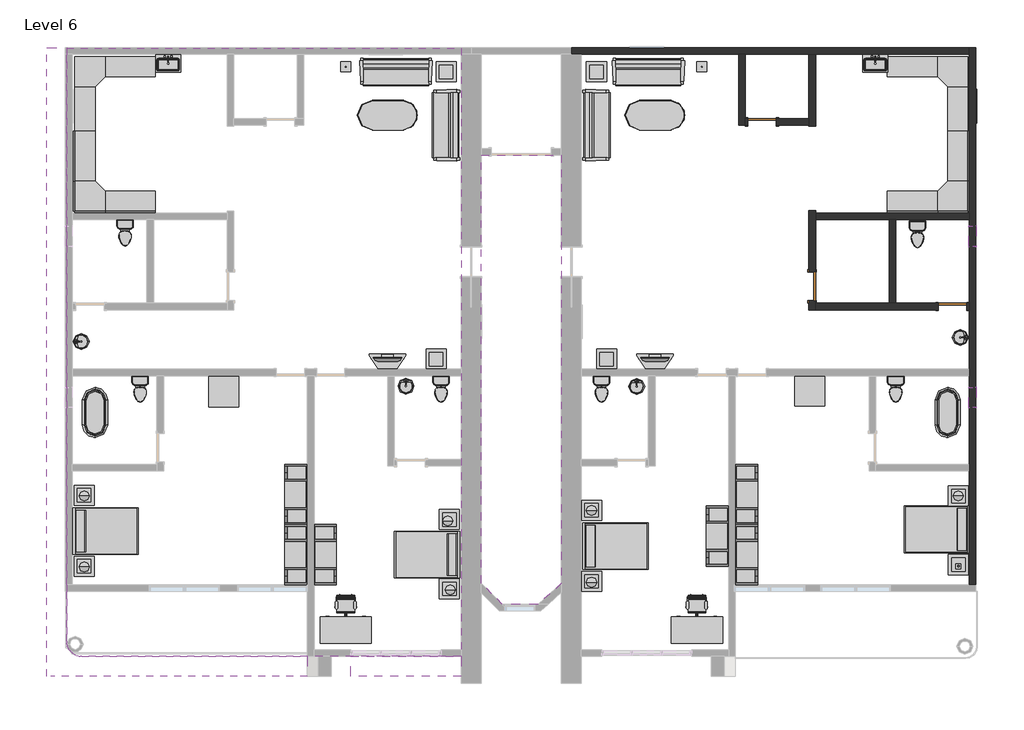
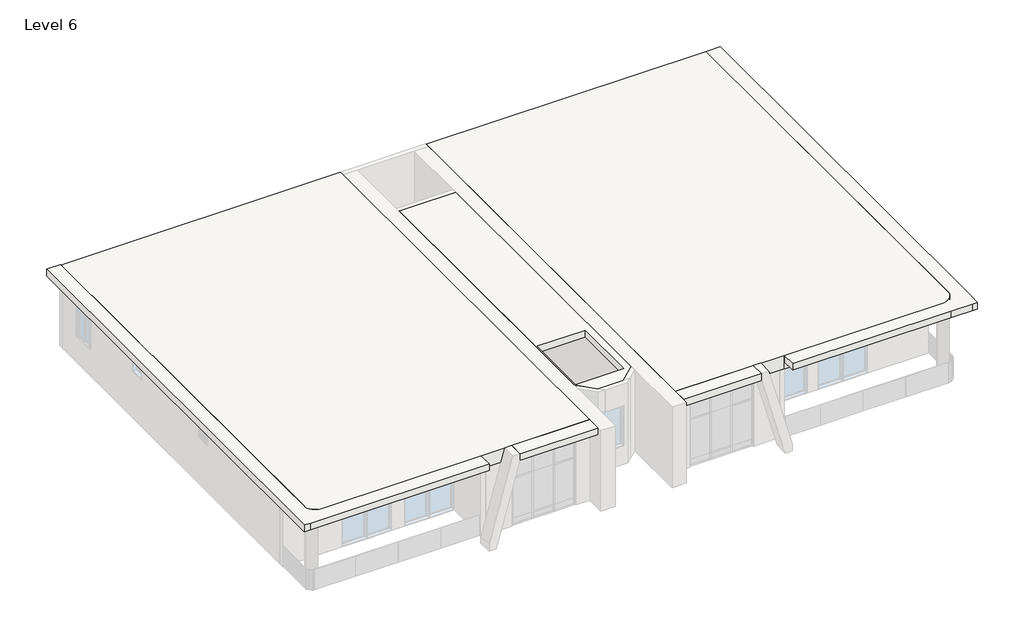
# One storey, part 3 of 3: 42 furniture elements, 14 flow terminals, 10 light fixtures, 9 walls, 4 slabs, 3 doors, 3 windows.
"""IFC4 building model written with IfcOpenShell, lengths in millimetres."""

from ifc_helpers import new_model, si_unit, point, frame, frame_2d, origin, place, context, project, spatial, polyline, circle_curve, trimmed, segment, composite_curve, outline, extrude, faceted_brep, transform, mapped, element, save
from components import door_2703ae13, door_10fd3a06, flow_terminal_38af2918, flow_terminal_d49f872f, toilet_domestic_3d_toilet_domestic_3d_f7549cf7, toilet_domestic_3d_toilet_domestic_3d_183bbd19, flow_terminal_b374fae2, furniture_07436f11, furniture_096e7f55, chair_task_arms_chair_task_arms_fa5a08ef, furniture_072f6425, furniture_cf0b6580, furniture_aff9b2fb, furniture_56245f3a, tv_stand_tv_stand_6ce107e5, furniture_b5c51a22, furniture_2c34a4f9, furniture_4d44e21c, furniture_45e3acac, light_fixture_100w_120v_8564026f, table_lamp_hemispheric_60w_120v_02721d88, window_0038ecf3, window_54100e87

model = new_model("IFC4")

# Units and contexts
model_context = context("Model", 3, world=origin())
ifc_project = project(units=[si_unit("LENGTHUNIT", "METRE", prefix="MILLI")], contexts=[model_context])

# Site, building, storey
site = spatial("IfcSite", under=ifc_project)
building = spatial("IfcBuilding", under=site)
storey = spatial("IfcBuildingStorey", under=building, Name="Level 6", Elevation=18288.0)

# Doors
placement = place(None, origin())
door_shape = door_2703ae13(model_context)
element("IfcDoor", 1, ObjectType="Door-Single-Panel.0001 : 34\" x 80\"", at=placement, inside=storey, context=model_context, shape_type="MappedRepresentation", body=[
    mapped(door_shape, transform((2522.0012296, 9464.0758558, 18288.0), x_axis=(-1.0, 0.0, 0.0), y_axis=(0.0, -1.0, 0.0), z_axis=(0.0, 0.0, 1.0))),
])
door_2_shape = door_10fd3a06(model_context)
element("IfcDoor", 2, ObjectType="Door-Single-Panel.0001 : 34\" x 80\"", at=placement, inside=storey, context=model_context, shape_type="MappedRepresentation", body=[
    mapped(door_2_shape, transform((8313.2012296, 3850.6758558, 18288.0), x_axis=(1.0, 0.0, 0.0), y_axis=(0.0, 1.0, 0.0), z_axis=(0.0, 0.0, 1.0))),
])
element("IfcDoor", 3, ObjectType="Door-Single-Panel.0001 : 34\" x 80\"", at=placement, inside=storey, context=model_context, shape_type="MappedRepresentation", body=[
    mapped(door_2_shape, transform((4046.0012296, 4460.2758558, 18288.0), x_axis=(0.0, -1.0, 0.0), y_axis=(1.0, 0.0, 0.0), z_axis=(0.0, 0.0, 1.0))),
])

# Flow terminals
flow_terminal_shape = flow_terminal_38af2918(model_context)
element("IfcFlowTerminal", 4, ObjectType="Sink Kitchen-Single : 30\" x 21\"", at=placement, inside=storey, context=model_context, shape_type="MappedRepresentation", body=[
    mapped(flow_terminal_shape, transform((-15540.388011, 11239.7304546, 18288.0), x_axis=(1.0, 0.0, 0.0), y_axis=(0.0, 1.0, 0.0), z_axis=(0.0, 0.0, 1.0))),
])
element("IfcFlowTerminal", 5, ObjectType="Sink Kitchen-Single : 30\" x 21\"", at=placement, inside=storey, context=model_context, shape_type="MappedRepresentation", body=[
    mapped(flow_terminal_shape, transform((5948.011989, 11239.7304546, 18288.0), x_axis=(1.0, 0.0, 0.0), y_axis=(0.0, 1.0, 0.0), z_axis=(0.0, 0.0, 1.0))),
])
flow_terminal_2_shape = flow_terminal_d49f872f(model_context)
element("IfcFlowTerminal", 6, ObjectType="Sink Vanity-Round : 19\" x 19\"", at=placement, inside=storey, context=model_context, shape_type="MappedRepresentation", body=[
    mapped(flow_terminal_2_shape, transform((-18084.6070794, 2687.2241152, 18288.0), x_axis=(0.0, 1.0, 0.0), y_axis=(-1.0, 0.0, 0.0), z_axis=(0.0, 0.0, 1.0))),
])
element("IfcFlowTerminal", 7, ObjectType="Sink Vanity-Round : 19\" x 19\"", at=placement, inside=storey, context=model_context, shape_type="MappedRepresentation", body=[
    mapped(flow_terminal_2_shape, transform((8462.2249463, 3007.5275963, 18288.0), x_axis=(0.0, -1.0, 0.0), y_axis=(1.0, 0.0, 0.0), z_axis=(0.0, 0.0, 1.0))),
])
element("IfcFlowTerminal", 8, ObjectType="Sink Vanity-Round : 19\" x 19\"", at=placement, inside=storey, context=model_context, shape_type="MappedRepresentation", body=[
    mapped(flow_terminal_2_shape, transform((-8395.050511, 1341.8921141, 18288.0), x_axis=(1.0, 0.0, 0.0), y_axis=(0.0, 1.0, 0.0), z_axis=(0.0, 0.0, 1.0))),
])
element("IfcFlowTerminal", 9, ObjectType="Sink Vanity-Round : 19\" x 19\"", at=placement, inside=storey, context=model_context, shape_type="MappedRepresentation", body=[
    mapped(flow_terminal_2_shape, transform((-1384.650511, 1331.0855344, 18288.0), x_axis=(1.0, 0.0, 0.0), y_axis=(0.0, 1.0, 0.0), z_axis=(0.0, 0.0, 1.0))),
])
toilet_domestic_3d_toilet_domestic_3d_shape = toilet_domestic_3d_toilet_domestic_3d_f7549cf7(model_context)
toilet_domestic_3d_toilet_domestic_3d_2_shape = toilet_domestic_3d_toilet_domestic_3d_183bbd19(model_context)
element("IfcFlowTerminal", 10, ObjectType="Toilet-Domestic-3D : Toilet-Domestic-3D", at=placement, inside=storey, context=model_context, shape_type="MappedRepresentation", body=[
    mapped(toilet_domestic_3d_toilet_domestic_3d_shape, transform((6586.0012296, 1247.7798284, 18288.0), x_axis=(1.0, 0.0, 0.0), y_axis=(0.0, 1.0, 0.0), z_axis=(0.0, 0.0, 1.0))),
    mapped(toilet_domestic_3d_toilet_domestic_3d_2_shape, transform((6586.0012296, 1247.7798284, 18288.0), x_axis=(1.0, 0.0, 0.0), y_axis=(0.0, 1.0, 0.0), z_axis=(0.0, 0.0, 1.0))),
])
element("IfcFlowTerminal", 11, ObjectType="Toilet-Domestic-3D : Toilet-Domestic-3D", at=placement, inside=storey, context=model_context, shape_type="MappedRepresentation", body=[
    mapped(toilet_domestic_3d_toilet_domestic_3d_shape, transform((-2354.7987704, 1247.7798284, 18288.0), x_axis=(1.0, 0.0, 0.0), y_axis=(0.0, 1.0, 0.0), z_axis=(0.0, 0.0, 1.0))),
    mapped(toilet_domestic_3d_toilet_domestic_3d_2_shape, transform((-2354.7987704, 1247.7798284, 18288.0), x_axis=(1.0, 0.0, 0.0), y_axis=(0.0, 1.0, 0.0), z_axis=(0.0, 0.0, 1.0))),
])
element("IfcFlowTerminal", 12, ObjectType="Toilet-Domestic-3D : Toilet-Domestic-3D", at=placement, inside=storey, context=model_context, shape_type="MappedRepresentation", body=[
    mapped(toilet_domestic_3d_toilet_domestic_3d_shape, transform((-16375.5987704, 1247.7798284, 18288.0), x_axis=(1.0, 0.0, 0.0), y_axis=(0.0, 1.0, 0.0), z_axis=(0.0, 0.0, 1.0))),
    mapped(toilet_domestic_3d_toilet_domestic_3d_2_shape, transform((-16375.5987704, 1247.7798284, 18288.0), x_axis=(1.0, 0.0, 0.0), y_axis=(0.0, 1.0, 0.0), z_axis=(0.0, 0.0, 1.0))),
])
element("IfcFlowTerminal", 13, ObjectType="Toilet-Domestic-3D : Toilet-Domestic-3D", at=placement, inside=storey, context=model_context, shape_type="MappedRepresentation", body=[
    mapped(toilet_domestic_3d_toilet_domestic_3d_shape, transform((-16832.7987704, 5997.5798284, 18288.0), x_axis=(1.0, 0.0, 0.0), y_axis=(0.0, 1.0, 0.0), z_axis=(0.0, 0.0, 1.0))),
    mapped(toilet_domestic_3d_toilet_domestic_3d_2_shape, transform((-16832.7987704, 5997.5798284, 18288.0), x_axis=(1.0, 0.0, 0.0), y_axis=(0.0, 1.0, 0.0), z_axis=(0.0, 0.0, 1.0))),
])
element("IfcFlowTerminal", 14, ObjectType="Toilet-Domestic-3D : Toilet-Domestic-3D", at=placement, inside=storey, context=model_context, shape_type="MappedRepresentation", body=[
    mapped(toilet_domestic_3d_toilet_domestic_3d_shape, transform((7246.4012296, 5946.7798284, 18288.0), x_axis=(1.0, 0.0, 0.0), y_axis=(0.0, 1.0, 0.0), z_axis=(0.0, 0.0, 1.0))),
    mapped(toilet_domestic_3d_toilet_domestic_3d_2_shape, transform((7246.4012296, 5946.7798284, 18288.0), x_axis=(1.0, 0.0, 0.0), y_axis=(0.0, 1.0, 0.0), z_axis=(0.0, 0.0, 1.0))),
])
element("IfcFlowTerminal", 15, ObjectType="Toilet-Domestic-3D : Toilet-Domestic-3D", at=placement, inside=storey, context=model_context, shape_type="MappedRepresentation", body=[
    mapped(toilet_domestic_3d_toilet_domestic_3d_shape, transform((-7231.5987704, 1247.7798284, 18288.0), x_axis=(1.0, 0.0, 0.0), y_axis=(0.0, 1.0, 0.0), z_axis=(0.0, 0.0, 1.0))),
    mapped(toilet_domestic_3d_toilet_domestic_3d_2_shape, transform((-7231.5987704, 1247.7798284, 18288.0), x_axis=(1.0, 0.0, 0.0), y_axis=(0.0, 1.0, 0.0), z_axis=(0.0, 0.0, 1.0))),
])
flow_terminal_3_shape = flow_terminal_b374fae2(model_context)
element("IfcFlowTerminal", 16, ObjectType="Tub-Free Standing-3D : 30\" x 60\"", at=placement, inside=storey, context=model_context, shape_type="MappedRepresentation", body=[
    mapped(flow_terminal_3_shape, transform((-17747.1987704, 624.8758558, 18288.0), x_axis=(1.0, 0.0, 0.0), y_axis=(0.0, 1.0, 0.0), z_axis=(0.0, 0.0, 1.0))),
])
element("IfcFlowTerminal", 17, ObjectType="Tub-Free Standing-3D : 30\" x 60\"", at=placement, inside=storey, context=model_context, shape_type="MappedRepresentation", body=[
    mapped(flow_terminal_3_shape, transform((8160.8012296, 624.8758558, 18288.0), x_axis=(1.0, 0.0, 0.0), y_axis=(0.0, 1.0, 0.0), z_axis=(0.0, 0.0, 1.0))),
])

# Furniture
furniture_shape = furniture_07436f11(model_context)
element("IfcFurniture", 18, ObjectType="96\" x 96\"", at=placement, inside=storey, context=model_context, shape_type="MappedRepresentation", body=[
    mapped(furniture_shape, transform((-18275.8670182, 11991.0988634, 18288.0), x_axis=(1.0, 0.0, 0.0), y_axis=(0.0, 1.0, 0.0), z_axis=(0.0, 0.0, 1.0))),
])
element("IfcFurniture", 19, ObjectType="96\" x 96\"", at=placement, inside=storey, context=model_context, shape_type="MappedRepresentation", body=[
    mapped(furniture_shape, transform((9316.2242372, 11364.3441035, 18288.0), x_axis=(0.0, -1.0, 0.0), y_axis=(1.0, 0.0, 0.0), z_axis=(0.0, 0.0, 1.0))),
])
furniture_2_shape = furniture_096e7f55(model_context)
element("IfcFurniture", 20, ObjectType="Bed-Shaker : Double 56\" x 78\"", at=placement, inside=storey, context=model_context, shape_type="MappedRepresentation", body=[
    mapped(furniture_2_shape, transform((-18407.5987704, -2962.8741442, 18288.0), x_axis=(0.0, 1.0, 0.0), y_axis=(-1.0, 0.0, 0.0), z_axis=(0.0, 0.0, 1.0))),
])
element("IfcFurniture", 21, ObjectType="Bed-Shaker : Double 56\" x 78\"", at=placement, inside=storey, context=model_context, shape_type="MappedRepresentation", body=[
    mapped(furniture_2_shape, transform((-6672.7987704, -3712.1741442, 18288.0), x_axis=(0.0, -1.0, 0.0), y_axis=(1.0, 0.0, 0.0), z_axis=(0.0, 0.0, 1.0))),
])
element("IfcFurniture", 22, ObjectType="Bed-Shaker : Double 56\" x 78\"", at=placement, inside=storey, context=model_context, shape_type="MappedRepresentation", body=[
    mapped(furniture_2_shape, transform((-2913.5987704, -3420.0741442, 18288.0), x_axis=(0.0, 1.0, 0.0), y_axis=(-1.0, 0.0, 0.0), z_axis=(0.0, 0.0, 1.0))),
])
element("IfcFurniture", 23, ObjectType="Bed-Shaker : Double 56\" x 78\"", at=placement, inside=storey, context=model_context, shape_type="MappedRepresentation", body=[
    mapped(furniture_2_shape, transform((8821.2012296, -2950.1741442, 18288.0), x_axis=(0.0, -1.0, 0.0), y_axis=(1.0, 0.0, 0.0), z_axis=(0.0, 0.0, 1.0))),
])
chair_task_arms_chair_task_arms_shape = chair_task_arms_chair_task_arms_fa5a08ef(model_context)
element("IfcFurniture", 24, ObjectType="Chair-Task Arms : Chair-Task Arms", at=placement, inside=storey, context=model_context, shape_type="MappedRepresentation", body=[
    mapped(chair_task_arms_chair_task_arms_shape, transform((681.7920493, -5184.3566833, 18288.0), x_axis=(-1.0, 0.0, 0.0), y_axis=(0.0, -1.0, 0.0), z_axis=(0.0, 0.0, 1.0))),
])
element("IfcFurniture", 25, ObjectType="Chair-Task Arms : Chair-Task Arms", at=placement, inside=storey, context=model_context, shape_type="MappedRepresentation", body=[
    mapped(chair_task_arms_chair_task_arms_shape, transform((-9986.2079507, -5184.3566833, 18288.0), x_axis=(-1.0, 0.0, 0.0), y_axis=(0.0, -1.0, 0.0), z_axis=(0.0, 0.0, 1.0))),
])
furniture_3_shape = furniture_072f6425(model_context)
element("IfcFurniture", 26, ObjectType="Desk : 60\" x 30\"", at=placement, inside=storey, context=model_context, shape_type="MappedRepresentation", body=[
    mapped(furniture_3_shape, transform((-10889.1987704, -6371.702585, 18288.0), x_axis=(1.0, 0.0, 0.0), y_axis=(0.0, 1.0, 0.0), z_axis=(0.0, 0.0, 1.0))),
])
element("IfcFurniture", 27, ObjectType="Desk : 60\" x 30\"", at=placement, inside=storey, context=model_context, shape_type="MappedRepresentation", body=[
    mapped(furniture_3_shape, transform((-221.1987704, -6371.702585, 18288.0), x_axis=(1.0, 0.0, 0.0), y_axis=(0.0, 1.0, 0.0), z_axis=(0.0, 0.0, 1.0))),
])
furniture_4_shape = furniture_cf0b6580(model_context)
element("IfcFurniture", 28, ObjectType="Entertainment Center : 72\" x 72\" x 24\"", at=placement, inside=storey, context=model_context, shape_type="MappedRepresentation", body=[
    mapped(furniture_4_shape, transform((1607.6012296, -3134.3241442, 18288.0), x_axis=(0.0, -1.0, 0.0), y_axis=(1.0, 0.0, 0.0), z_axis=(0.0, 0.0, 1.0))),
])
element("IfcFurniture", 29, ObjectType="Entertainment Center : 72\" x 72\" x 24\"", at=placement, inside=storey, context=model_context, shape_type="MappedRepresentation", body=[
    mapped(furniture_4_shape, transform((1607.6012296, -3693.1241442, 18288.0), x_axis=(0.0, 1.0, 0.0), y_axis=(-1.0, 0.0, 0.0), z_axis=(0.0, 0.0, 1.0))),
])
element("IfcFurniture", 30, ObjectType="Entertainment Center : 72\" x 72\" x 24\"", at=placement, inside=storey, context=model_context, shape_type="MappedRepresentation", body=[
    mapped(furniture_4_shape, transform((1607.6012296, -1864.3241442, 18288.0), x_axis=(0.0, 1.0, 0.0), y_axis=(-1.0, 0.0, 0.0), z_axis=(0.0, 0.0, 1.0))),
])
element("IfcFurniture", 31, ObjectType="Entertainment Center : 72\" x 72\" x 24\"", at=placement, inside=storey, context=model_context, shape_type="MappedRepresentation", body=[
    mapped(furniture_4_shape, transform((-11193.9987704, -3693.1241442, 18288.0), x_axis=(0.0, -1.0, 0.0), y_axis=(1.0, 0.0, 0.0), z_axis=(0.0, 0.0, 1.0))),
])
element("IfcFurniture", 32, ObjectType="Entertainment Center : 72\" x 72\" x 24\"", at=placement, inside=storey, context=model_context, shape_type="MappedRepresentation", body=[
    mapped(furniture_4_shape, transform((-11193.9987704, -1864.3241442, 18288.0), x_axis=(0.0, -1.0, 0.0), y_axis=(1.0, 0.0, 0.0), z_axis=(0.0, 0.0, 1.0))),
])
element("IfcFurniture", 33, ObjectType="Entertainment Center : 72\" x 72\" x 24\"", at=placement, inside=storey, context=model_context, shape_type="MappedRepresentation", body=[
    mapped(furniture_4_shape, transform((-11193.9987704, -3693.1241442, 18288.0), x_axis=(0.0, 1.0, 0.0), y_axis=(-1.0, 0.0, 0.0), z_axis=(0.0, 0.0, 1.0))),
])
furniture_5_shape = furniture_aff9b2fb(model_context)
element("IfcFurniture", 34, ObjectType="Sofa-Pensi : 84\"", at=placement, inside=storey, context=model_context, shape_type="MappedRepresentation", body=[
    mapped(furniture_5_shape, transform((-8881.8050204, 10710.9660197, 18288.0), x_axis=(1.0, 0.0, 0.0), y_axis=(0.0, 1.0, 0.0), z_axis=(0.0, 0.0, 1.0))),
])
element("IfcFurniture", 35, ObjectType="Sofa-Pensi : 84\"", at=placement, inside=storey, context=model_context, shape_type="MappedRepresentation", body=[
    mapped(furniture_5_shape, transform((-7356.3086065, 9641.0821058, 18288.0), x_axis=(0.0, -1.0, 0.0), y_axis=(1.0, 0.0, 0.0), z_axis=(0.0, 0.0, 1.0))),
])
element("IfcFurniture", 36, ObjectType="Sofa-Pensi : 84\"", at=placement, inside=storey, context=model_context, shape_type="MappedRepresentation", body=[
    mapped(furniture_5_shape, transform((-2230.0889343, 9083.8696058, 18288.0), x_axis=(0.0, 1.0, 0.0), y_axis=(-1.0, 0.0, 0.0), z_axis=(0.0, 0.0, 1.0))),
])
element("IfcFurniture", 37, ObjectType="Sofa-Pensi : 84\"", at=placement, inside=storey, context=model_context, shape_type="MappedRepresentation", body=[
    mapped(furniture_5_shape, transform((-1211.0050204, 10710.9660197, 18288.0), x_axis=(1.0, 0.0, 0.0), y_axis=(0.0, 1.0, 0.0), z_axis=(0.0, 0.0, 1.0))),
])
furniture_6_shape = furniture_56245f3a(model_context)
element("IfcFurniture", 38, ObjectType="TV - Flat Screen : 32\"", at=placement, inside=storey, context=model_context, shape_type="MappedRepresentation", body=[
    mapped(furniture_6_shape, transform((-8861.1432846, 2232.8144794, 19202.4), x_axis=(-1.0, 0.0, 0.0), y_axis=(0.0, -1.0, 0.0), z_axis=(0.0, 0.0, 1.0))),
])
element("IfcFurniture", 39, ObjectType="TV - Flat Screen : 32\"", at=placement, inside=storey, context=model_context, shape_type="MappedRepresentation", body=[
    mapped(furniture_6_shape, transform((-733.1432846, 2232.8144794, 19202.4), x_axis=(-1.0, 0.0, 0.0), y_axis=(0.0, -1.0, 0.0), z_axis=(0.0, 0.0, 1.0))),
])
tv_stand_tv_stand_shape = tv_stand_tv_stand_6ce107e5(model_context)
element("IfcFurniture", 40, ObjectType="TV Stand : TV Stand", at=placement, inside=storey, context=model_context, shape_type="MappedRepresentation", body=[
    mapped(tv_stand_tv_stand_shape, transform((-8732.0107683, 1945.6758558, 18288.0), x_axis=(-1.0, 0.0, 0.0), y_axis=(0.0, -1.0, 0.0), z_axis=(0.0, 0.0, 1.0))),
])
element("IfcFurniture", 41, ObjectType="TV Stand : TV Stand", at=placement, inside=storey, context=model_context, shape_type="MappedRepresentation", body=[
    mapped(tv_stand_tv_stand_shape, transform((-604.0107683, 1945.6758558, 18288.0), x_axis=(-1.0, 0.0, 0.0), y_axis=(0.0, -1.0, 0.0), z_axis=(0.0, 0.0, 1.0))),
])
furniture_7_shape = furniture_b5c51a22(model_context)
element("IfcFurniture", 42, ObjectType="Table-Coffee : 24\" x 24\" x 24\"", at=placement, inside=storey, context=model_context, shape_type="MappedRepresentation", body=[
    mapped(furniture_7_shape, transform((-7097.4645371, 10892.864778, 18288.0), x_axis=(1.0, 0.0, 0.0), y_axis=(0.0, 1.0, 0.0), z_axis=(0.0, 0.0, 1.0))),
])
element("IfcFurniture", 43, ObjectType="Table-Coffee : 24\" x 24\" x 24\"", at=placement, inside=storey, context=model_context, shape_type="MappedRepresentation", body=[
    mapped(furniture_7_shape, transform((-2525.4645371, 10892.864778, 18288.0), x_axis=(1.0, 0.0, 0.0), y_axis=(0.0, 1.0, 0.0), z_axis=(0.0, 0.0, 1.0))),
])
element("IfcFurniture", 44, ObjectType="Table-Coffee : 24\" x 24\" x 24\"", at=placement, inside=storey, context=model_context, shape_type="MappedRepresentation", body=[
    mapped(furniture_7_shape, transform((-7402.2645371, 2155.264778, 18288.0), x_axis=(1.0, 0.0, 0.0), y_axis=(0.0, 1.0, 0.0), z_axis=(0.0, 0.0, 1.0))),
])
element("IfcFurniture", 45, ObjectType="Table-Coffee : 24\" x 24\" x 24\"", at=placement, inside=storey, context=model_context, shape_type="MappedRepresentation", body=[
    mapped(furniture_7_shape, transform((-2220.6645371, 2155.264778, 18288.0), x_axis=(1.0, 0.0, 0.0), y_axis=(0.0, 1.0, 0.0), z_axis=(0.0, 0.0, 1.0))),
])
element("IfcFurniture", 46, ObjectType="Table-Coffee : 24\" x 24\" x 24\"", at=placement, inside=storey, context=model_context, shape_type="MappedRepresentation", body=[
    mapped(furniture_7_shape, transform((-2677.8645371, -4601.135222, 18288.0), x_axis=(1.0, 0.0, 0.0), y_axis=(0.0, 1.0, 0.0), z_axis=(0.0, 0.0, 1.0))),
])
element("IfcFurniture", 47, ObjectType="Table-Coffee : 24\" x 24\" x 24\"", at=placement, inside=storey, context=model_context, shape_type="MappedRepresentation", body=[
    mapped(furniture_7_shape, transform((-18095.6645371, -4143.935222, 18288.0), x_axis=(1.0, 0.0, 0.0), y_axis=(0.0, 1.0, 0.0), z_axis=(0.0, 0.0, 1.0))),
])
element("IfcFurniture", 48, ObjectType="Table-Coffee : 24\" x 24\" x 24\"", at=placement, inside=storey, context=model_context, shape_type="MappedRepresentation", body=[
    mapped(furniture_7_shape, transform((-18095.6645371, -1984.935222, 18288.0), x_axis=(1.0, 0.0, 0.0), y_axis=(0.0, 1.0, 0.0), z_axis=(0.0, 0.0, 1.0))),
])
element("IfcFurniture", 49, ObjectType="Table-Coffee : 24\" x 24\" x 24\"", at=placement, inside=storey, context=model_context, shape_type="MappedRepresentation", body=[
    mapped(furniture_7_shape, transform((-2677.8645371, -2442.135222, 18288.0), x_axis=(1.0, 0.0, 0.0), y_axis=(0.0, 1.0, 0.0), z_axis=(0.0, 0.0, 1.0))),
])
element("IfcFurniture", 50, ObjectType="Table-Coffee : 24\" x 24\" x 24\"", at=placement, inside=storey, context=model_context, shape_type="MappedRepresentation", body=[
    mapped(furniture_7_shape, transform((8472.7354629, -4093.135222, 18288.0), x_axis=(1.0, 0.0, 0.0), y_axis=(0.0, 1.0, 0.0), z_axis=(0.0, 0.0, 1.0))),
])
element("IfcFurniture", 51, ObjectType="Table-Coffee : 24\" x 24\" x 24\"", at=placement, inside=storey, context=model_context, shape_type="MappedRepresentation", body=[
    mapped(furniture_7_shape, transform((8472.7354629, -2010.335222, 18288.0), x_axis=(1.0, 0.0, 0.0), y_axis=(0.0, 1.0, 0.0), z_axis=(0.0, 0.0, 1.0))),
])
element("IfcFurniture", 52, ObjectType="Table-Coffee : 24\" x 24\" x 24\"", at=placement, inside=storey, context=model_context, shape_type="MappedRepresentation", body=[
    mapped(furniture_7_shape, transform((-6995.8645371, -4832.0414601, 18288.0), x_axis=(1.0, 0.0, 0.0), y_axis=(0.0, 1.0, 0.0), z_axis=(0.0, 0.0, 1.0))),
])
element("IfcFurniture", 53, ObjectType="Table-Coffee : 24\" x 24\" x 24\"", at=placement, inside=storey, context=model_context, shape_type="MappedRepresentation", body=[
    mapped(furniture_7_shape, transform((-6995.8645371, -2723.8414601, 18288.0), x_axis=(1.0, 0.0, 0.0), y_axis=(0.0, 1.0, 0.0), z_axis=(0.0, 0.0, 1.0))),
])
furniture_8_shape = furniture_2c34a4f9(model_context)
element("IfcFurniture", 54, ObjectType="Table-Dining Oval : 36\" x 72\"", at=placement, inside=storey, context=model_context, shape_type="MappedRepresentation", body=[
    mapped(furniture_8_shape, transform((-8455.3790983, 10025.3742164, 18288.0), x_axis=(1.0, 0.0, 0.0), y_axis=(0.0, 1.0, 0.0), z_axis=(0.0, 0.0, 1.0))),
])
element("IfcFurniture", 55, ObjectType="Table-Dining Oval : 36\" x 72\"", at=placement, inside=storey, context=model_context, shape_type="MappedRepresentation", body=[
    mapped(furniture_8_shape, transform((-327.3790983, 10025.3742164, 18288.0), x_axis=(1.0, 0.0, 0.0), y_axis=(0.0, 1.0, 0.0), z_axis=(0.0, 0.0, 1.0))),
])
furniture_9_shape = furniture_4d44e21c(model_context)
element("IfcFurniture", 56, ObjectType="Table-Rectangular : 36\" x 36\"", at=placement, inside=storey, context=model_context, shape_type="MappedRepresentation", body=[
    mapped(furniture_9_shape, transform((-13835.5987704, 1259.8758558, 18288.0), x_axis=(1.0, 0.0, 0.0), y_axis=(0.0, 1.0, 0.0), z_axis=(0.0, 0.0, 1.0))),
])
element("IfcFurniture", 57, ObjectType="Table-Rectangular : 36\" x 36\"", at=placement, inside=storey, context=model_context, shape_type="MappedRepresentation", body=[
    mapped(furniture_9_shape, transform((3969.8012296, 1285.2758558, 18288.0), x_axis=(1.0, 0.0, 0.0), y_axis=(0.0, 1.0, 0.0), z_axis=(0.0, 0.0, 1.0))),
])
furniture_10_shape = furniture_45e3acac(model_context)
element("IfcFurniture", 58, ObjectType="Work Station Cubicle : 96\" x 96\"", at=placement, inside=storey, context=model_context, shape_type="MappedRepresentation", body=[
    mapped(furniture_10_shape, transform((-18902.621778, 6827.207608, 18288.0), x_axis=(0.0, 1.0, 0.0), y_axis=(-1.0, 0.0, 0.0), z_axis=(0.0, 0.0, 1.0))),
])
element("IfcFurniture", 59, ObjectType="Work Station Cubicle : 96\" x 96\"", at=placement, inside=storey, context=model_context, shape_type="MappedRepresentation", body=[
    mapped(furniture_10_shape, transform((8689.4694774, 6200.4528481, 18288.0), x_axis=(-1.0, 0.0, 0.0), y_axis=(0.0, -1.0, 0.0), z_axis=(0.0, 0.0, 1.0))),
])

# Light fixtures
light_fixture_100w_120v_shape = light_fixture_100w_120v_8564026f(model_context)
element("IfcLightFixture", 60, ObjectType="100W - 120V", at=placement, inside=storey, context=model_context, shape_type="MappedRepresentation", body=[
    mapped(light_fixture_100w_120v_shape, transform((-10127.1987704, 11140.4758558, 18288.0), x_axis=(1.0, 0.0, 0.0), y_axis=(0.0, 1.0, 0.0), z_axis=(0.0, 0.0, 1.0))),
])
element("IfcLightFixture", 61, ObjectType="100W - 120V", at=placement, inside=storey, context=model_context, shape_type="MappedRepresentation", body=[
    mapped(light_fixture_100w_120v_shape, transform((693.2012296, 11140.4758558, 18288.0), x_axis=(1.0, 0.0, 0.0), y_axis=(0.0, 1.0, 0.0), z_axis=(0.0, 0.0, 1.0))),
])
table_lamp_hemispheric_60w_120v_shape = table_lamp_hemispheric_60w_120v_02721d88(model_context)
element("IfcLightFixture", 62, ObjectType="Table Lamp - Hemispheric : 60W - 120V", at=placement, inside=storey, context=model_context, shape_type="MappedRepresentation", body=[
    mapped(table_lamp_hemispheric_60w_120v_shape, transform((-18077.3987704, -1915.1241442, 18897.6), x_axis=(1.0, 0.0, 0.0), y_axis=(0.0, 1.0, 0.0), z_axis=(0.0, 0.0, 1.0))),
])
element("IfcLightFixture", 63, ObjectType="Table Lamp - Hemispheric : 60W - 120V", at=placement, inside=storey, context=model_context, shape_type="MappedRepresentation", body=[
    mapped(table_lamp_hemispheric_60w_120v_shape, transform((-7028.3987704, -2666.7303823, 18897.6), x_axis=(1.0, 0.0, 0.0), y_axis=(0.0, 1.0, 0.0), z_axis=(0.0, 0.0, 1.0))),
])
element("IfcLightFixture", 64, ObjectType="Table Lamp - Hemispheric : 60W - 120V", at=placement, inside=storey, context=model_context, shape_type="MappedRepresentation", body=[
    mapped(table_lamp_hemispheric_60w_120v_shape, transform((-2659.5987704, -2346.9241442, 18897.6), x_axis=(1.0, 0.0, 0.0), y_axis=(0.0, 1.0, 0.0), z_axis=(0.0, 0.0, 1.0))),
])
element("IfcLightFixture", 65, ObjectType="Table Lamp - Hemispheric : 60W - 120V", at=placement, inside=storey, context=model_context, shape_type="MappedRepresentation", body=[
    mapped(table_lamp_hemispheric_60w_120v_shape, transform((8491.0012296, -4048.7241442, 19202.4), x_axis=(1.0, 0.0, 0.0), y_axis=(0.0, 1.0, 0.0), z_axis=(0.0, 0.0, 1.0))),
])
element("IfcLightFixture", 66, ObjectType="Table Lamp - Hemispheric : 60W - 120V", at=placement, inside=storey, context=model_context, shape_type="MappedRepresentation", body=[
    mapped(table_lamp_hemispheric_60w_120v_shape, transform((8491.0012296, -1915.1241442, 18897.6), x_axis=(1.0, 0.0, 0.0), y_axis=(0.0, 1.0, 0.0), z_axis=(0.0, 0.0, 1.0))),
])
element("IfcLightFixture", 67, ObjectType="Table Lamp - Hemispheric : 60W - 120V", at=placement, inside=storey, context=model_context, shape_type="MappedRepresentation", body=[
    mapped(table_lamp_hemispheric_60w_120v_shape, transform((-2659.5987704, -4531.3241442, 18897.6), x_axis=(1.0, 0.0, 0.0), y_axis=(0.0, 1.0, 0.0), z_axis=(0.0, 0.0, 1.0))),
])
element("IfcLightFixture", 68, ObjectType="Table Lamp - Hemispheric : 60W - 120V", at=placement, inside=storey, context=model_context, shape_type="MappedRepresentation", body=[
    mapped(table_lamp_hemispheric_60w_120v_shape, transform((-6952.1987704, -4762.2303823, 18897.6), x_axis=(1.0, 0.0, 0.0), y_axis=(0.0, 1.0, 0.0), z_axis=(0.0, 0.0, 1.0))),
])
element("IfcLightFixture", 69, ObjectType="Table Lamp - Hemispheric : 60W - 120V", at=placement, inside=storey, context=model_context, shape_type="MappedRepresentation", body=[
    mapped(table_lamp_hemispheric_60w_120v_shape, transform((-18077.3987704, -4074.1241442, 18897.6), x_axis=(1.0, 0.0, 0.0), y_axis=(0.0, 1.0, 0.0), z_axis=(0.0, 0.0, 1.0))),
])

# Slabs
element("IfcSlab", 70, ObjectType="Generic - 12\" cream", at=placement, inside=storey, context=model_context, shape_type="SweptSolid", body=[
    extrude(outline(composite_curve([segment(polyline([(-6621.9987704, 11699.2758558), (-6621.9987704, -6791.9241442), (-11295.5987704, -6791.9241442), (-18153.5987704, -6791.9241442)]), True, "CONTINUOUS"), segment(trimmed(circle_curve(frame_2d((-18153.5987704, -6334.7241442)), 457.2), [point((-18153.5987704, -6791.9241442))], [point((-18610.7987704, -6334.7241442))], False, "CARTESIAN"), True, "CONTINUOUS"), segment(polyline([(-18610.7987704, -6334.7241442), (-18610.7987704, 11699.2758558), (-6621.9987704, 11699.2758558)]), True, "CONTINUOUS")], self_intersect=False)), frame((0.0, 0.0, 21336.0), z_axis=(0.0, 0.0, 1.0), x_axis=(1.0, 0.0, 0.0)), (0.0, 0.0, 1.0), 609.6),
    extrude(outline(composite_curve([segment(trimmed(circle_curve(frame_2d((8511.8043381, -6277.3874522)), 514.536692), [point((9024.4012296, -6322.0241442))], [point((8511.8043381, -6791.9241442))], False, "CARTESIAN"), True, "CONTINUOUS"), segment(polyline([(8511.8043381, -6791.9241442), (1709.2012296, -6791.9241442), (-2862.7987704, -6791.9241442), (-2964.3987704, -6791.9241442), (-2964.3987704, 11699.2758558), (9024.4012296, 11699.2758558), (9024.4012296, -6322.0241442)]), True, "CONTINUOUS")], self_intersect=False)), frame((0.0, 0.0, 21336.0), z_axis=(0.0, 0.0, 1.0), x_axis=(1.0, 0.0, 0.0)), (0.0, 0.0, 1.0), 609.6),
])
element("IfcSlab", 71, ObjectType="Generic - 12\" white", at=placement, inside=storey, context=model_context, shape_type="SweptSolid", body=[
    extrude(outline(composite_curve([segment(polyline([(9634.0012296, 11699.2758558), (9634.0012296, -6931.6241442), (9634.0012296, -7401.5241442), (9430.8012296, -7401.5241442), (8511.8043381, -7401.5241442), (1709.2012296, -7401.5241442), (1709.2012296, -6791.9241442), (8511.8043381, -6791.9241442)]), True, "CONTINUOUS"), segment(trimmed(circle_curve(frame_2d((8511.8043381, -6277.3874522)), 514.536692), [point((8511.8043381, -6791.9241442))], [point((9024.4012296, -6322.0241442))], True, "CARTESIAN"), True, "CONTINUOUS"), segment(polyline([(9024.4012296, -6322.0241442), (9024.4012296, 11699.2758558), (9634.0012296, 11699.2758558)]), True, "CONTINUOUS")], self_intersect=False)), frame((0.0, 0.0, 21640.8), z_axis=(0.0, 0.0, 1.0), x_axis=(1.0, 0.0, 0.0)), (0.0, 0.0, 1.0), 304.8),
    extrude(outline(composite_curve([segment(polyline([(-18610.7987704, 11724.6758558), (-18610.7987704, -6334.7241442)]), True, "CONTINUOUS"), segment(trimmed(circle_curve(frame_2d((-18153.5987704, -6334.7241442)), 457.2), [point((-18610.7987704, -6334.7241442))], [point((-18153.5987704, -6791.9241442))], True, "CARTESIAN"), True, "CONTINUOUS"), segment(polyline([(-18153.5987704, -6791.9241442), (-11295.5987704, -6791.9241442), (-11295.5987704, -7401.5241442), (-18966.3987704, -7401.5241442), (-19220.3987704, -7401.5241442), (-19220.3987704, 11724.6758558), (-18610.7987704, 11724.6758558)]), True, "CONTINUOUS")], self_intersect=False)), frame((0.0, 0.0, 21640.8), z_axis=(0.0, 0.0, 1.0), x_axis=(1.0, 0.0, 0.0)), (0.0, 0.0, 1.0), 304.8),
])
element("IfcSlab", 72, ObjectType="Generic - 12\" white", at=placement, inside=storey, context=model_context, shape_type="SweptSolid", body=[
    extrude(outline(polyline([(387.8709824, -6791.9241442), (387.8709824, -7401.5241442), (-2958.0487704, -7401.5241442), (-2958.0487704, -6791.9241442), (387.8709824, -6791.9241442)])), frame((0.0, 0.0, 21640.8), z_axis=(0.0, 0.0, 1.0), x_axis=(1.0, 0.0, 0.0)), (0.0, 0.0, 1.0), 304.8),
    extrude(outline(polyline([(-9974.7987704, -6791.9241442), (-6615.6487704, -6791.9241442), (-6615.6487704, -7401.5241442), (-9974.7987704, -7401.5241442), (-9974.7987704, -6791.9241442)])), frame((0.0, 0.0, 21640.8), z_axis=(0.0, 0.0, 1.0), x_axis=(1.0, 0.0, 0.0)), (0.0, 0.0, 1.0), 304.8),
])
element("IfcSlab", 73, ObjectType="Generic - 12\" white", at=placement, inside=storey, context=model_context, shape_type="SweptSolid", body=[
    extrude(outline(polyline([(-3573.9987704, 8448.0758558), (-3573.9987704, -1691.5549149), (-3573.9987704, -4572.9908503), (-4280.7801413, -5203.302585), (-5372.9801413, -5203.302585), (-6006.858582, -4569.4241442), (-6006.858582, -1692.8741442), (-6006.0487704, -1692.8741442), (-6006.0487704, 8448.0758558), (-3573.9987704, 8448.0758558)]), holes=[polyline([(-5940.8822214, -4561.7549149), (-3883.4822214, -4561.7549149), (-3883.4822214, -1691.5549149), (-5940.8822214, -1691.5549149), (-5940.8822214, -4561.7549149)])]), frame((0.0, 0.0, 21640.8), z_axis=(0.0, 0.0, 1.0), x_axis=(1.0, 0.0, 0.0)), (0.0, 0.0, 1.0), 304.8),
])

# Walls
element("IfcWall", 74, ObjectType="Generic - 8\" cream", at=placement, inside=storey, context=model_context, shape_type="Brep", body=[
    faceted_brep([(8821.2012296, 11724.6758558, 18288.0), (8821.2012296, 11521.4758558, 18288.0), (8821.2012296, 6695.4758558, 18288.0), (8821.2012296, 6492.2758558, 18288.0), (8821.2012296, 3952.2758558, 18288.0), (8821.2012296, 3749.0758558, 18288.0), (8821.2012296, 1945.6758558, 18288.0), (8821.2012296, 1742.4758558, 18288.0), (8821.2012296, -949.9241442, 18288.0), (8821.2012296, -1153.1241442, 18288.0), (8821.2012296, -4607.5241442, 18288.0), (8821.2012296, -4607.5241442, 21336.0), (8821.2012296, -1153.1241442, 21336.0), (8821.2012296, -949.9241442, 21336.0), (8821.2012296, 1742.4758558, 21336.0), (8821.2012296, 1945.6758558, 21336.0), (8821.2012296, 3749.0758558, 21336.0), (8821.2012296, 3952.2758558, 21336.0), (8821.2012296, 6492.2758558, 21336.0), (8821.2012296, 6695.4758558, 21336.0), (8821.2012296, 11521.4758558, 21336.0), (8821.2012296, 11724.6758558, 21336.0), (8821.2012296, 10403.8758558, 19507.2), (8821.2012296, 10403.8758558, 20726.4), (8821.2012296, 9489.4758558, 20726.4), (8821.2012296, 9489.4758558, 19507.2), (8821.2012296, 777.2758558, 21031.2), (8821.2012296, 777.2758558, 20421.6), (8821.2012296, 1386.8758558, 20421.6), (8821.2012296, 1386.8758558, 21031.2), (8821.2012296, 6289.0758558, 20421.6), (8821.2012296, 6289.0758558, 21031.2), (8821.2012296, 5679.4758558, 21031.2), (8821.2012296, 5679.4758558, 20421.6), (9024.4012296, -4607.5241442, 18288.0), (9024.4012296, 11724.6758558, 18288.0), (9024.4012296, 11724.6758558, 21336.0), (9024.4012296, -4607.5241442, 21336.0), (9024.4012296, 10403.8758558, 20726.4), (9024.4012296, 10403.8758558, 19507.2), (9024.4012296, 9489.4758558, 19507.2), (9024.4012296, 9489.4758558, 20726.4), (9024.4012296, 777.2758558, 20421.6), (9024.4012296, 777.2758558, 21031.2), (9024.4012296, 1386.8758558, 21031.2), (9024.4012296, 1386.8758558, 20421.6), (9024.4012296, 6289.0758558, 21031.2), (9024.4012296, 6289.0758558, 20421.6), (9024.4012296, 5679.4758558, 20421.6), (9024.4012296, 5679.4758558, 21031.2)], [[[0, 1, 2, 3, 4, 5, 6, 7, 8, 9, 10, 11, 12, 13, 14, 15, 16, 17, 18, 19, 20, 21], [22, 23, 24, 25], [26, 27, 28, 29], [30, 31, 32, 33]], [[34, 35, 36, 37], [38, 39, 40, 41], [42, 43, 44, 45], [46, 47, 48, 49]], [[10, 9, 8, 7, 6, 5, 4, 3, 2, 1, 0, 35, 34]], [[21, 20, 19, 18, 17, 16, 15, 14, 13, 12, 11, 37, 36]], [[0, 21, 36, 35]], [[11, 10, 34, 37]], [[39, 38, 23, 22]], [[40, 39, 22, 25]], [[41, 40, 25, 24]], [[38, 41, 24, 23]], [[26, 43, 42, 27]], [[27, 42, 45, 28]], [[28, 45, 44, 29]], [[43, 26, 29, 44]], [[46, 31, 30, 47]], [[47, 30, 33, 48]], [[48, 33, 32, 49]], [[31, 46, 49, 32]]]),
])
element("IfcWall", 75, ObjectType="Generic - 8\" cream", at=placement, inside=storey, context=model_context, shape_type="Brep", body=[
    faceted_brep([(3944.4012296, 11521.4758558, 18288.0), (3944.4012296, 9565.6758558, 18288.0), (3944.4012296, 9362.4758558, 18288.0), (3944.4012296, 9337.0758558, 18288.0), (3944.4012296, 9337.0758558, 21336.0), (3944.4012296, 9362.4758558, 21336.0), (3944.4012296, 9565.6758558, 21336.0), (3944.4012296, 11521.4758558, 21336.0), (4147.6012296, 11521.4758558, 18288.0), (4147.6012296, 11521.4758558, 21336.0), (4147.6012296, 9337.0758558, 21336.0), (4147.6012296, 9337.0758558, 18288.0)], [[[0, 1, 2, 3, 4, 5, 6, 7]], [[8, 9, 10, 11]], [[3, 2, 1, 0, 8, 11]], [[4, 3, 11, 10]], [[7, 6, 5, 4, 10, 9]], [[0, 7, 9, 8]]]),
])
element("IfcWall", 76, ObjectType="Generic - 8\" cream", at=placement, inside=storey, context=model_context, shape_type="Brep", body=[
    faceted_brep([(4147.6012296, 6492.2758558, 18288.0), (6382.8012296, 6492.2758558, 18288.0), (6586.0012296, 6492.2758558, 18288.0), (8821.2012296, 6492.2758558, 18288.0), (8821.2012296, 6492.2758558, 21336.0), (6586.0012296, 6492.2758558, 21336.0), (6382.8012296, 6492.2758558, 21336.0), (4147.6012296, 6492.2758558, 21336.0), (4147.6012296, 6695.4758558, 18288.0), (4147.6012296, 6695.4758558, 21336.0), (8821.2012296, 6695.4758558, 21336.0), (8821.2012296, 6695.4758558, 18288.0)], [[[0, 1, 2, 3, 4, 5, 6, 7]], [[8, 9, 10, 11]], [[3, 2, 1, 0, 8, 11]], [[7, 6, 5, 4, 10, 9]], [[0, 7, 9, 8]], [[4, 3, 11, 10]]]),
])
element("IfcWall", 77, ObjectType="Generic - 8\" cream", at=placement, inside=storey, context=model_context, shape_type="Brep", body=[
    faceted_brep([(8821.2012296, 3749.0758558, 21336.0), (4147.6012296, 3749.0758558, 21336.0), (4147.6012296, 3749.0758558, 18288.0), (7881.4012296, 3749.0758558, 18288.0), (7881.4012296, 3749.0758558, 20320.0), (8745.0012296, 3749.0758558, 20320.0), (8745.0012296, 3749.0758558, 18288.0), (8821.2012296, 3749.0758558, 18288.0), (4147.6012296, 3952.2758558, 21336.0), (6382.8012296, 3952.2758558, 21336.0), (6586.0012296, 3952.2758558, 21336.0), (8821.2012296, 3952.2758558, 21336.0), (8821.2012296, 3952.2758558, 18288.0), (8745.0012296, 3952.2758558, 18288.0), (8745.0012296, 3952.2758558, 20320.0), (7881.4012296, 3952.2758558, 20320.0), (7881.4012296, 3952.2758558, 18288.0), (6586.0012296, 3952.2758558, 18288.0), (6382.8012296, 3952.2758558, 18288.0), (4147.6012296, 3952.2758558, 18288.0)], [[[0, 1, 2, 3, 4, 5, 6, 7]], [[8, 9, 10, 11, 12, 13, 14, 15, 16, 17, 18, 19]], [[2, 19, 18, 17, 16, 3]], [[12, 7, 6, 13]], [[1, 0, 11, 10, 9, 8]], [[2, 1, 8, 19]], [[0, 7, 12, 11]], [[5, 14, 13, 6]], [[14, 5, 4, 15]], [[15, 4, 3, 16]]]),
])
element("IfcWall", 78, ObjectType="Generic - 8\" cream", at=placement, inside=storey, context=model_context, shape_type="SweptSolid", body=[
    extrude(outline(polyline([(21336.0, 3944.4012296), (21336.0, 2014.0012296), (18288.0, 2014.0012296), (18288.0, 2090.2012296), (20320.0, 2090.2012296), (20320.0, 2953.8012296), (18288.0, 2953.8012296), (18288.0, 3944.4012296), (21336.0, 3944.4012296)])), frame((0.0, 9362.4758558, 0.0), z_axis=(0.0, 1.0, 0.0), x_axis=(0.0, 0.0, 1.0)), (0.0, 0.0, 1.0), 203.2),
])
element("IfcWall", 79, ObjectType="Generic - 8\" cream", at=placement, inside=storey, context=model_context, shape_type="SweptSolid", body=[
    extrude(outline(polyline([(6382.8012296, 3952.2758558), (6382.8012296, 6492.2758558), (6586.0012296, 6492.2758558), (6586.0012296, 3952.2758558), (6382.8012296, 3952.2758558)])), frame((0.0, 0.0, 18288.0), z_axis=(0.0, 0.0, 1.0), x_axis=(1.0, 0.0, 0.0)), (0.0, 0.0, 1.0), 3048.0),
])
element("IfcWall", 80, ObjectType="Generic - 8\" cream", at=placement, inside=storey, context=model_context, shape_type="Brep", body=[
    faceted_brep([(3944.4012296, 3749.0758558, 21336.0), (3944.4012296, 6771.6758558, 21336.0), (3944.4012296, 6771.6758558, 18288.0), (3944.4012296, 4892.0758558, 18288.0), (3944.4012296, 4892.0758558, 20320.0), (3944.4012296, 4028.4758558, 20320.0), (3944.4012296, 4028.4758558, 18288.0), (3944.4012296, 3749.0758558, 18288.0), (4147.6012296, 6771.6758558, 21336.0), (4147.6012296, 6695.4758558, 21336.0), (4147.6012296, 6492.2758558, 21336.0), (4147.6012296, 3952.2758558, 21336.0), (4147.6012296, 3749.0758558, 21336.0), (4147.6012296, 3749.0758558, 18288.0), (4147.6012296, 3952.2758558, 18288.0), (4147.6012296, 4028.4758558, 18288.0), (4147.6012296, 4028.4758558, 20320.0), (4147.6012296, 4892.0758558, 20320.0), (4147.6012296, 4892.0758558, 18288.0), (4147.6012296, 6492.2758558, 18288.0), (4147.6012296, 6695.4758558, 18288.0), (4147.6012296, 6771.6758558, 18288.0)], [[[0, 1, 2, 3, 4, 5, 6, 7]], [[8, 9, 10, 11, 12, 13, 14, 15, 16, 17, 18, 19, 20, 21]], [[2, 21, 20, 19, 18, 3]], [[13, 7, 6, 15, 14]], [[1, 0, 12, 11, 10, 9, 8]], [[2, 1, 8, 21]], [[0, 7, 13, 12]], [[5, 16, 15, 6]], [[16, 5, 4, 17]], [[17, 4, 3, 18]]]),
])
element("IfcWall", 81, ObjectType="Generic - 8\" cream", at=placement, inside=storey, context=model_context, shape_type="Brep", body=[
    faceted_brep([(-3269.1987704, 11521.4758558, 18288.0), (-2964.3987704, 11521.4758558, 18288.0), (1810.8012296, 11521.4758558, 18288.0), (2014.0012296, 11521.4758558, 18288.0), (3944.4012296, 11521.4758558, 18288.0), (4147.6012296, 11521.4758558, 18288.0), (8821.2012296, 11521.4758558, 18288.0), (8821.2012296, 11521.4758558, 21336.0), (4147.6012296, 11521.4758558, 21336.0), (3944.4012296, 11521.4758558, 21336.0), (2014.0012296, 11521.4758558, 21336.0), (1810.8012296, 11521.4758558, 21336.0), (-2964.3987704, 11521.4758558, 21336.0), (-3269.1987704, 11521.4758558, 21336.0), (-1440.3987704, 11521.4758558, 20726.4), (-525.9987704, 11521.4758558, 20726.4), (-525.9987704, 11521.4758558, 19507.2), (-1440.3987704, 11521.4758558, 19507.2), (-3269.1987704, 11724.6758558, 18288.0), (-3269.1987704, 11724.6758558, 21336.0), (-2964.3987704, 11724.6758558, 21336.0), (8821.2012296, 11724.6758558, 21336.0), (8821.2012296, 11724.6758558, 18288.0), (-1440.3987704, 11724.6758558, 20726.4), (-1440.3987704, 11724.6758558, 19507.2), (-525.9987704, 11724.6758558, 19507.2), (-525.9987704, 11724.6758558, 20726.4)], [[[0, 1, 2, 3, 4, 5, 6, 7, 8, 9, 10, 11, 12, 13], [14, 15, 16, 17]], [[18, 19, 20, 21, 22], [23, 24, 25, 26]], [[6, 5, 4, 3, 2, 1, 0, 18, 22]], [[13, 12, 11, 10, 9, 8, 7, 21, 20, 19]], [[0, 13, 19, 18]], [[7, 6, 22, 21]], [[23, 26, 15, 14]], [[26, 25, 16, 15]], [[25, 24, 17, 16]], [[24, 23, 14, 17]]]),
])
element("IfcWall", 82, ObjectType="Generic - 8\" white", at=placement, inside=storey, context=model_context, shape_type="Brep", body=[
    faceted_brep([(1810.8012296, 11521.4758558, 18288.0), (1810.8012296, 9362.4758558, 18288.0), (1810.8012296, 9362.4758558, 21336.0), (1810.8012296, 11521.4758558, 21336.0), (2014.0012296, 11521.4758558, 18288.0), (2014.0012296, 11521.4758558, 21336.0), (2014.0012296, 9565.6758558, 21336.0), (2014.0012296, 9362.4758558, 21336.0), (2014.0012296, 9362.4758558, 18288.0), (2014.0012296, 9565.6758558, 18288.0)], [[[0, 1, 2, 3]], [[4, 5, 6, 7, 8, 9]], [[1, 0, 4, 9, 8]], [[3, 2, 7, 6, 5]], [[0, 3, 5, 4]], [[2, 1, 8, 7]]]),
])

# Windows
window_shape = window_0038ecf3(model_context)
element("IfcWindow", 83, ObjectType="Louvers with Trim : 24\" x 24\"", at=placement, inside=storey, context=model_context, shape_type="MappedRepresentation", body=[
    mapped(window_shape, transform((8916.4512296, 5984.2758558, 19507.2), x_axis=(0.0, 1.0, 0.0), y_axis=(-1.0, 0.0, 0.0), z_axis=(0.0, 0.0, 1.0))),
])
element("IfcWindow", 84, ObjectType="Louvers with Trim : 24\" x 24\"", at=placement, inside=storey, context=model_context, shape_type="MappedRepresentation", body=[
    mapped(window_shape, transform((8929.1512296, 1082.0758558, 19507.2), x_axis=(0.0, -1.0, 0.0), y_axis=(1.0, 0.0, 0.0), z_axis=(0.0, 0.0, 1.0))),
])
window_2_shape = window_54100e87(model_context)
element("IfcWindow", 85, ObjectType="Slider with Trim : 36\" x 48\"", at=placement, inside=storey, context=model_context, shape_type="MappedRepresentation", body=[
    mapped(window_2_shape, transform((8922.8012296, 9946.6758558, 18592.8), x_axis=(0.0, 1.0, 0.0), y_axis=(-1.0, 0.0, 0.0), z_axis=(0.0, 0.0, 1.0))),
])

save(model, "model.ifc")

# Revit data of these elements
# Type "Door-Single-Panel.0001 : 34\" x 80\""
#   Type Mark = "9"
#   Construction Type Id = "DOOR"
#   Assembly Code = "C1020300"
#   Analytic Construction = "Wooden"
#   Thickness = 0' - 2"
#   Thermal Resistance (R) = 0.455703 (m²·K)/W
#   Swing Angle [instance default] = 90.00°
#   Heat Transfer Coefficient (U) = 2.19465 W/(m²·K)
#   Height = 6' - 8"
#   Trim Projection Ext = 0' - 1"
#   Trim Projection Int = 0' - 1"
#   Trim Width = 0' - 3"
#   Width = 2' - 10"
#   Panel Material = Wood - Birch - Solid Stained Light Low Gloss
#   Trim Material = Paint - Sienna
#   Visual Light Transmittance = 0
#   Solar Heat Gain Coefficient = 0
#   Function = (empty or 0)
#   Wall Closure = (empty or 0)
# Type "Sink Kitchen-Single : 30\" x 21\""
#   Assembly Code = "D2010410"
#   Counter Height = 3' - 0"
#   Depth = 1' - 9"
#   Width = 2' - 6"
#   Faucet Material = Steel, Polished
#   Sink Material = Steel, Polished
# Type "Sink Vanity-Round : 19\" x 19\""
#   Assembly Code = "D2010400"
#   Top Of Counter = 2' - 7"
#   Basin Material = Porcelain, Linen
#   Faucet Material = Steel, Polished
# Type "Toilet-Domestic-3D : Toilet-Domestic-3D"
#   Assembly Code = "D2010110"
#   Toilet - Bowl/Basin Material = Porcelain, Linen
#   Toilet - Seat Material = Laminate, Linen, Matte
# Type "Tub-Free Standing-3D : 30\" x 60\""
#   Assembly Code = "D2010110"
#   Height = 1' - 6"
#   Length = 5' - 0"
#   Width = 2' - 6"
#   Tub Material = Porcelain, Ivory
# Type "96\" x 96\""
#   Assembly Code = "E2020"
#   Desktop Height = 2' - 6"
#   Desktop1 Width = 2' - 0"
#   Desktop2 Width = 2' - 0"
#   Panel1 Length = 5' - 0"
#   Panel2 Length = 5' - 0"
#   Work Top Material = Laminate, Ivory, Matte
# Type "Bed-Shaker : Double 56\" x 78\""
#   Assembly Code = "E2020200"
#   Length = 6' - 6"
#   Width = 4' - 8"
#   Frame Material = Birch
#   Mattress Material = Linen, White
# Type "Chair-Task Arms : Chair-Task Arms"
#   Assembly Code = "E2020200"
#   Base Material = Plastic, Opaque Black
#   Caster Material = Plastic, Opaque Black
#   Seat/Back Material = Textile - Slate Blue
# Type "Desk : 60\" x 30\""
#   Assembly Code = "E2020200"
#   Depth = 2' - 6"
#   Height = 2' - 6"
#   Leg Height = 0' - 6"
#   Width = 5' - 0"
#   Body Material = Laminate, Ivory, Matte
#   Handle/Leg Material = Steel, Chrome Plated
#   Top Material = Cherry
# Type "Entertainment Center : 72\" x 72\" x 24\""
#   Assembly Code = "E2020200"
#   Center Width = 2' - 8"
#   Depth = 2' - 0"
#   Height = 6' - 0"
#   Width = 6' - 0"
#   Material = none
# Type "Sofa-Pensi : 84\""
#   Assembly Code = "E2020200"
#   Length = 7' - 0"
#   Frame Material = Cherry
#   Seat Material = Linen, Beige
#   Feet Material = Steel, Chrome Plated
# Type "TV - Flat Screen : 32\""
#   SinAng = 0' - 0.0193"
#   L = 2' - 3.79372"
#   H = 1' - 3.6354"
#   Thickness = 0' - 4.33071"
#   Diagonal = 2' - 7.88976"
#   CosAng = 0' - 0.03431"
#   Stand [instance default] = yes
# Type "TV Stand : TV Stand"
#   Depth = 1' - 6"
#   Width = 3' - 8"
#   Height = 1' - 7 1/2"
#   Finish = Melamine - Gray
# Type "Table-Coffee : 24\" x 24\" x 24\""
#   Assembly Code = "E2020200"
#   Height = 2' - 0"
#   Length = 2' - 0"
#   Width = 2' - 0"
#   Top Material = none
#   Frame Material = none
# Type "Table-Dining Oval : 36\" x 72\""
#   Assembly Code = "E2020200"
#   Length = 6' - 0"
#   Width = 3' - 0"
#   Base Material = Steel, Chrome Plated
#   Top Material = Glass - Clear, Grey
#   Description = (empty or 0)
# Type "Table-Rectangular : 36\" x 36\""
#   Assembly Code = "E2020200"
#   Height = 2' - 6"
#   Length = 3' - 0"
#   Width = 3' - 0"
#   Base Material = Birch
#   Top Material = Birch
# Type "Work Station Cubicle : 96\" x 96\""
#   Assembly Code = "E2020"
#   Desktop Height = 2' - 6"
#   Desktop1 Width = 2' - 0"
#   Desktop2 Width = 2' - 0"
#   Panel Height = 5' - 6"
#   Panel1 Length = 5' - 0"
#   Panel2 Length = 5' - 0"
#   Cube Panel Material = Textile - Light Gray
#   Work Top Material = Laminate, Ivory, Matte
# Type "100W - 120V"
#   Assembly Code = "D5020220"
#   Lamp = "A-19"
#   Wattage Comments = "100"
#   Wattage = 100 W
#   built-in parameter 1150110 = 1 (stored number, unit not read)
#   built-in parameter 1114217 = 1 (stored number, unit not read)
#   built-in parameter 1150109 = 1 (stored number, unit not read)
#   built-in parameter 1150113 = 1 (stored number, unit not read)
#   built-in parameter 1150115 = 1 (stored number, unit not read)
#   built-in parameter 1150105 = 139.261 (stored number, unit not read)
#   Light Source Symbol Size = 2' - 0"
#   built-in parameter 1150112 = 1 (stored number, unit not read)
#   built-in parameter 1150114 = 1 (stored number, unit not read)
#   built-in parameter 1150107 = 2800 (stored number, unit not read)
#   built-in parameter 1150106 = 1.39261 (stored number, unit not read)
#   built-in parameter 1150104 = 1.6258 (stored number, unit not read)
#   Ballast Voltage = 120 V
#   built-in parameter 1114218 = 1 (stored number, unit not read)
#   built-in parameter 1150133 = 10 (stored number, unit not read)
#   Lumens = 1750 lm
#   Apparent Load = 100 VA
#   built-in parameter 1150134 = 4
#   built-in parameter 1150137 = 1
#   Color Filter = 16777215
#   Ballast Number of Poles = 1
#   Shade = Glass, Frosted
#   Stand = Steel, Chrome Plated
#   Dimming Lamp Color Temperature Shift = (empty or 0)
# Type "Table Lamp - Hemispheric : 60W - 120V"
#   Assembly Code = "D5020220"
#   Lamp = "A-19"
#   Wattage = 60 W
#   built-in parameter 1150110 = 1 (stored number, unit not read)
#   built-in parameter 1114217 = 1 (stored number, unit not read)
#   built-in parameter 1150109 = 1 (stored number, unit not read)
#   built-in parameter 1150113 = 1 (stored number, unit not read)
#   built-in parameter 1150115 = 1 (stored number, unit not read)
#   built-in parameter 1150105 = 68.0387 (stored number, unit not read)
#   Light Source Symbol Size = 2' - 0"
#   built-in parameter 1150112 = 1 (stored number, unit not read)
#   built-in parameter 1150114 = 1 (stored number, unit not read)
#   built-in parameter 1150107 = 2800 (stored number, unit not read)
#   built-in parameter 1150106 = 0.680387 (stored number, unit not read)
#   built-in parameter 1150104 = 1.32387 (stored number, unit not read)
#   Ballast Voltage = 120 V
#   built-in parameter 1114218 = 1 (stored number, unit not read)
#   built-in parameter 1150133 = 10 (stored number, unit not read)
#   Lumens = 855 lm
#   Apparent Load = 60 VA
#   built-in parameter 1150134 = 4
#   built-in parameter 1150137 = 1
#   Color Filter = 16777215
#   Ballast Number of Poles = 1
#   Mount Material = Steel, Chrome Plated
#   Shade Material = Glass, Frosted
#   Base Material = Birch
#   Dimming Lamp Color Temperature Shift = (empty or 0)
#   Wattage Comments = ""
# Type "Generic - 12\" cream"
#   Assembly Code = "B1010"
#   Thickness = 2' - 0"
#   Function = 0
#   Layers, outside or top first: 2' - 0" "Parking Stripe" (function 1)
# Type "Generic - 12\" white"
#   Assembly Code = "B1010"
#   Thickness = 1' - 0"
#   Function = 0
#   Layers, outside or top first: 1' - 0" "Door - Frame" (function 1)
# Type "Generic - 8\" cream"
#   Assembly Code = "B2010"
#   Width = 0' - 8"
#   Layers, outside or top first: 0' - 8" "Parking Stripe" (function 1)
# Type "Generic - 8\" white"
#   Assembly Code = "B2010"
#   Width = 0' - 8"
#   Layers, outside or top first: 0' - 8" "Door - Frame" (function 1)
# Type "Louvers with Trim : 24\" x 24\""
#   Type Mark = "27"
#   Construction Type Id = "GSP4R"
#   Assembly Code = "B20"
#   Analytic Construction = "1/8 in Pilkington single glazing"
#   Visual Light Transmittance = 0.9
#   Solar Heat Gain Coefficient = 0.78
#   Heat Transfer Coefficient (U) = 3.6886 W/(m²·K)
#   Default Sill Height = 3' - 0"
#   Trim Projection - Ext. = 0' - 0 1/2"
#   Trim Projection - Int. = 0' - 0 1/2"
#   Trim Width - Exterior = 0' - 1 1/2"
#   Trim Width - Interior = 0' - 1 1/2"
#   Width = 2' - 0"
#   Frame Material = Iron, Ductile
#   Louver Material = Glass
#   Trim Exterior Material = Glass
#   Trim Interior Material = Iron, Ductile
#   Wall Closure = (empty or 0)
# Type "Slider with Trim : 36\" x 48\""
#   Type Mark = "11"
#   Construction Type Id = "GSP4R"
#   Assembly Code = "B2020100"
#   Analytic Construction = "1/8 in Pilkington single glazing"
#   Visual Light Transmittance = 0.9
#   Solar Heat Gain Coefficient = 0.78
#   Heat Transfer Coefficient (U) = 3.6886 W/(m²·K)
#   Height = 4' - 0"
#   Default Sill Height = 3' - 0"
#   Trim Projection - Ext. = 0' - 0 3/4"
#   Trim Projection - Int. = 0' - 0 3/4"
#   Trim Width - Exterior = 0' - 3 1/2"
#   Trim Width - Interior = 0' - 3 1/2"
#   Width = 3' - 0"
#   Window Inset = 0' - 0 3/4"
#   Glass Pane Material = Glass
#   Sash Material = Iron, Ductile
#   Trim Exterior Material = Iron, Ductile
#   Trim Interior Material = Iron, Ductile
#   Wall Closure = (empty or 0)
# Elements 1, 2, 3 (IfcDoor, "Door-Single-Panel.0001 : 34\" x 80\"")
#   Swing Angle = 90.00°
#   Phase Created = New Construction
#   Materials on its faces: "Paint - Sienna", "Wood - Birch - Solid Stained Light Low Gloss"
# Element 4 (IfcFlowTerminal, "Sink Kitchen-Single : 30\" x 21\"")
#   Mark = "95"
#   Phase Created = New Construction
#   Materials on its faces: "Steel, Polished"
# Element 5 (IfcFlowTerminal, "Sink Kitchen-Single : 30\" x 21\"")
#   Mark = "96"
#   Phase Created = New Construction
#   Materials on its faces: "Steel, Polished"
# Element 6 (IfcFlowTerminal, "Sink Vanity-Round : 19\" x 19\"")
#   Mark = "99"
#   Phase Created = New Construction
#   Materials on its faces: "Porcelain, Linen", "Steel, Polished"
# Element 7 (IfcFlowTerminal, "Sink Vanity-Round : 19\" x 19\"")
#   Mark = "100"
#   Phase Created = New Construction
#   Materials on its faces: "Porcelain, Linen", "Steel, Polished"
# Element 8 (IfcFlowTerminal, "Sink Vanity-Round : 19\" x 19\"")
#   Mark = "107"
#   Phase Created = New Construction
#   Materials on its faces: "Porcelain, Linen", "Steel, Polished"
# Element 9 (IfcFlowTerminal, "Sink Vanity-Round : 19\" x 19\"")
#   Mark = "108"
#   Phase Created = New Construction
#   Materials on its faces: "Porcelain, Linen", "Steel, Polished"
# Element 10 (IfcFlowTerminal, "Toilet-Domestic-3D : Toilet-Domestic-3D")
#   Mark = "101"
#   Phase Created = New Construction
#   Materials on its faces: "Porcelain, Linen", "Laminate, Linen, Matte"
# Element 11 (IfcFlowTerminal, "Toilet-Domestic-3D : Toilet-Domestic-3D")
#   Mark = "102"
#   Phase Created = New Construction
#   Materials on its faces: "Porcelain, Linen", "Laminate, Linen, Matte"
# Element 12 (IfcFlowTerminal, "Toilet-Domestic-3D : Toilet-Domestic-3D")
#   Mark = "103"
#   Phase Created = New Construction
#   Materials on its faces: "Porcelain, Linen", "Laminate, Linen, Matte"
# Element 13 (IfcFlowTerminal, "Toilet-Domestic-3D : Toilet-Domestic-3D")
#   Mark = "104"
#   Phase Created = New Construction
#   Materials on its faces: "Porcelain, Linen", "Laminate, Linen, Matte"
# Element 14 (IfcFlowTerminal, "Toilet-Domestic-3D : Toilet-Domestic-3D")
#   Mark = "105"
#   Phase Created = New Construction
#   Materials on its faces: "Porcelain, Linen", "Laminate, Linen, Matte"
# Element 15 (IfcFlowTerminal, "Toilet-Domestic-3D : Toilet-Domestic-3D")
#   Mark = "106"
#   Phase Created = New Construction
#   Materials on its faces: "Porcelain, Linen", "Laminate, Linen, Matte"
# Element 16 (IfcFlowTerminal, "Tub-Free Standing-3D : 30\" x 60\"")
#   Mark = "93"
#   Phase Created = New Construction
#   Materials on its faces: "Porcelain, Ivory"
# Element 17 (IfcFlowTerminal, "Tub-Free Standing-3D : 30\" x 60\"")
#   Mark = "94"
#   Phase Created = New Construction
#   Materials on its faces: "Porcelain, Ivory"
# Elements 18, 19 (IfcFurniture, "96\" x 96\"")
#   Phase Created = New Construction
#   Materials on its faces: "Laminate, Ivory, Matte"
# Elements 20, 21, 22, 23 (IfcFurniture, "Bed-Shaker : Double 56\" x 78\"")
#   Phase Created = New Construction
#   Materials on its faces: "Birch", "Linen, White"
# Elements 24, 25 (IfcFurniture, "Chair-Task Arms : Chair-Task Arms")
#   Phase Created = New Construction
#   Materials on its faces: "Plastic, Opaque Black", "Textile - Slate Blue"
